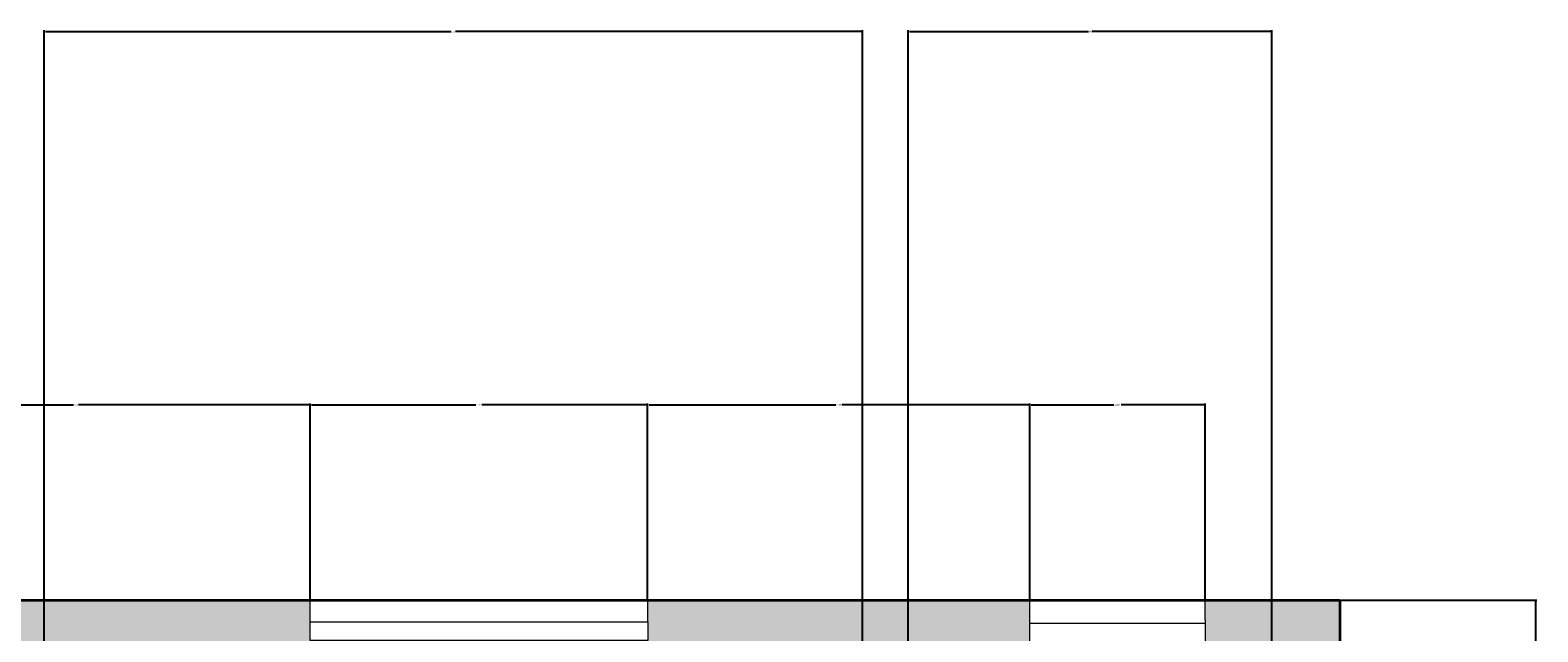
# Model space of a CAD drawing. Units: inches. Extents: x 3024 to 3952, y 1308 to 1863.
# Tile 27 of 29: x 3297 to 3496, y 1783 to 1863. Entities that reach past the tile are written whole.
import ezdxf

# ---------------------------------------------------------------- set-up
doc = ezdxf.new("R2010")
doc.units = ezdxf.units.IN
for name, color, linetype, lineweight in [('A-ANNO-DIMS', 2, 'Continuous', 18), ('A-GLAZ', 4, 'Continuous', 18), ('A-WALL', 7, 'Continuous', 35)]:
    doc.layers.add(name, color=color, linetype=linetype, lineweight=lineweight)
doc.layers.add('A-WALL-PATT', color=254, linetype='Continuous', lineweight=13, true_color=0xcecce6)
doc.styles.get("Standard").update_dxf_attribs({"font": 'arial.ttf'})
doc.dimstyles.get("Standard").update_dxf_attribs({"dimtxt": 0.18, "dimasz": 0.18, "dimexe": 0.18, "dimexo": 0.0625, "dimgap": 0.09, "dimtad": 0, "dimtih": 1, "dimtoh": 1, "dimdec": 4, "dimzin": 0, "dimdsep": 46, "dimtxsty": 'Standard', "dimcen": 0.09, "dimadec": 0, "dimazin": 0, "dimtfac": 1, "dimtdec": 4, "dimtofl": 0, "dimtmove": 0, "dimatfit": 3, "dimfxl": 1, "dimtolj": 1, "dimtzin": 0, "dimarcsym": 0})

# ---------------------------------------------------------------- blocks, each defined once
blk = doc.blocks.new('*D37')
at = {"layer": 'A-ANNO-DIMS', "color": 0, "lineweight": -2, "transparency": 16777216}
for p, q in [((3469.83, 1787.61), (3495.72, 1787.61)), ((3495.54, 1787.43), (3495.54, 1567.91)), ((3495.54, 1348.03), (3495.54, 1567.54)), ((3469.83, 1347.85), (3495.72, 1347.85))]:
    blk.add_line(p, q, dxfattribs=at)
at = {"layer": 'A-ANNO-DIMS', "color": 0, "transparency": 16777216}
for points in [[(3495.51, 1787.43), (3495.57, 1787.43), (3495.54, 1787.61)], [(3495.51, 1348.03), (3495.57, 1348.03), (3495.54, 1347.85)]]:
    blk.add_solid(points, dxfattribs=at)
at = {"layer": 'Defpoints', "color": 0, "transparency": 16777216}
for p in [(3469.76, 1787.61), (3495.54, 1787.61), (3469.76, 1347.85)]:
    blk.add_point(p, dxfattribs=at)
at = {"layer": 'A-ANNO-DIMS', "color": 0, "transparency": 16777216, "insert": (3495.54, 1567.73), "char_height": 0.18, "attachment_point": 5}
blk.add_mtext('\\A1;439.8', dxfattribs=at)
blk = doc.blocks.new('*D40')
at = {"layer": 'A-ANNO-DIMS', "color": 0, "lineweight": -2, "transparency": 16777216}
for p, q in [((3298.76, 1778.67), (3298.76, 1862.78)), ((3298.94, 1862.6), (3352.48, 1862.6)), ((3406.58, 1862.6), (3353.04, 1862.6)), ((3406.76, 1778.67), (3406.76, 1862.78))]:
    blk.add_line(p, q, dxfattribs=at)
at = {"layer": 'A-ANNO-DIMS', "color": 0, "transparency": 16777216}
for points in [[(3298.94, 1862.63), (3298.94, 1862.57), (3298.76, 1862.6)], [(3406.58, 1862.63), (3406.58, 1862.57), (3406.76, 1862.6)]]:
    blk.add_solid(points, dxfattribs=at)
at = {"layer": 'Defpoints', "color": 0, "transparency": 16777216}
for p in [(3406.76, 1862.6), (3298.76, 1778.61), (3406.76, 1778.61)]:
    blk.add_point(p, dxfattribs=at)
at = {"layer": 'A-ANNO-DIMS', "color": 0, "transparency": 16777216, "insert": (3352.76, 1862.6), "char_height": 0.18, "attachment_point": 5}
blk.add_mtext('\\A1;108', dxfattribs=at)
blk = doc.blocks.new('*D41')
at = {"layer": 'A-ANNO-DIMS', "color": 0, "lineweight": -2, "transparency": 16777216}
for p, q in [((3412.76, 1778.67), (3412.76, 1862.78)), ((3412.94, 1862.6), (3436.54, 1862.6)), ((3460.58, 1862.6), (3436.99, 1862.6)), ((3460.76, 1778.67), (3460.76, 1862.78))]:
    blk.add_line(p, q, dxfattribs=at)
at = {"layer": 'A-ANNO-DIMS', "color": 0, "transparency": 16777216}
for points in [[(3412.94, 1862.63), (3412.94, 1862.57), (3412.76, 1862.6)], [(3460.58, 1862.63), (3460.58, 1862.57), (3460.76, 1862.6)]]:
    blk.add_solid(points, dxfattribs=at)
at = {"layer": 'Defpoints', "color": 0, "transparency": 16777216}
for p in [(3460.76, 1862.6), (3412.76, 1778.61), (3460.76, 1778.61)]:
    blk.add_point(p, dxfattribs=at)
at = {"layer": 'A-ANNO-DIMS', "color": 0, "transparency": 16777216, "insert": (3436.76, 1862.6), "char_height": 0.18, "attachment_point": 5}
blk.add_mtext('\\A1;48', dxfattribs=at)
blk = doc.blocks.new('*D69')
at = {"layer": 'A-ANNO-DIMS', "color": 0, "lineweight": -2, "transparency": 16777216}
for p, q in [((3333.86, 1787.67), (3333.86, 1813.56)), ((3334.04, 1813.38), (3355.73, 1813.38)), ((3378.21, 1813.38), (3356.52, 1813.38)), ((3378.39, 1787.67), (3378.39, 1813.56))]:
    blk.add_line(p, q, dxfattribs=at)
at = {"layer": 'A-ANNO-DIMS', "color": 0, "transparency": 16777216}
for points in [[(3334.04, 1813.41), (3334.04, 1813.35), (3333.86, 1813.38)], [(3378.21, 1813.41), (3378.21, 1813.35), (3378.39, 1813.38)]]:
    blk.add_solid(points, dxfattribs=at)
at = {"layer": 'Defpoints', "color": 0, "transparency": 16777216}
for p in [(3378.39, 1813.38), (3333.86, 1787.61), (3378.39, 1787.61)]:
    blk.add_point(p, dxfattribs=at)
at = {"layer": 'A-ANNO-DIMS', "color": 0, "transparency": 16777216, "insert": (3356.13, 1813.38), "char_height": 0.18, "attachment_point": 5}
blk.add_mtext('\\A1;44.54', dxfattribs=at)
blk = doc.blocks.new('*D70')
at = {"layer": 'A-ANNO-DIMS', "color": 0, "lineweight": -2, "transparency": 16777216}
for p, q in [((3428.83, 1787.67), (3428.83, 1813.56)), ((3429.01, 1813.38), (3439.92, 1813.38)), ((3451.76, 1813.38), (3440.85, 1813.38)), ((3451.94, 1787.67), (3451.94, 1813.56))]:
    blk.add_line(p, q, dxfattribs=at)
at = {"layer": 'A-ANNO-DIMS', "color": 0, "transparency": 16777216}
for points in [[(3429.01, 1813.41), (3429.01, 1813.35), (3428.83, 1813.38)], [(3451.76, 1813.41), (3451.76, 1813.35), (3451.94, 1813.38)]]:
    blk.add_solid(points, dxfattribs=at)
at = {"layer": 'Defpoints', "color": 0, "transparency": 16777216}
for p in [(3451.94, 1813.38), (3428.83, 1787.61), (3451.94, 1787.61)]:
    blk.add_point(p, dxfattribs=at)
at = {"layer": 'A-ANNO-DIMS', "color": 0, "transparency": 16777216, "insert": (3440.39, 1813.38), "char_height": 0.18, "attachment_point": 5}
blk.add_mtext('\\A1;23.104', dxfattribs=at)
blk = doc.blocks.new('*D73')
at = {"layer": 'A-ANNO-DIMS', "color": 0, "lineweight": -2, "transparency": 16777216}
for p, q in [((3272.05, 1787.67), (3272.05, 1813.56)), ((3272.23, 1813.38), (3302.63, 1813.38)), ((3333.68, 1813.38), (3303.28, 1813.38)), ((3333.86, 1787.67), (3333.86, 1813.56))]:
    blk.add_line(p, q, dxfattribs=at)
at = {"layer": 'A-ANNO-DIMS', "color": 0, "transparency": 16777216}
for points in [[(3272.23, 1813.41), (3272.23, 1813.35), (3272.05, 1813.38)], [(3333.68, 1813.41), (3333.68, 1813.35), (3333.86, 1813.38)]]:
    blk.add_solid(points, dxfattribs=at)
at = {"layer": 'Defpoints', "color": 0, "transparency": 16777216}
for p in [(3333.86, 1813.38), (3272.05, 1787.61), (3333.86, 1787.61)]:
    blk.add_point(p, dxfattribs=at)
at = {"layer": 'A-ANNO-DIMS', "color": 0, "transparency": 16777216, "insert": (3302.95, 1813.38), "char_height": 0.18, "attachment_point": 5}
blk.add_mtext('\\A1;61.8', dxfattribs=at)
blk = doc.blocks.new('*D74')
at = {"layer": 'A-ANNO-DIMS', "color": 0, "lineweight": -2, "transparency": 16777216}
for p, q in [((3378.39, 1787.67), (3378.39, 1813.56)), ((3378.57, 1813.38), (3403.22, 1813.38)), ((3428.65, 1813.38), (3404.01, 1813.38)), ((3428.83, 1787.67), (3428.83, 1813.56))]:
    blk.add_line(p, q, dxfattribs=at)
at = {"layer": 'A-ANNO-DIMS', "color": 0, "transparency": 16777216}
for points in [[(3378.57, 1813.41), (3378.57, 1813.35), (3378.39, 1813.38)], [(3428.65, 1813.41), (3428.65, 1813.35), (3428.83, 1813.38)]]:
    blk.add_solid(points, dxfattribs=at)
at = {"layer": 'Defpoints', "color": 0, "transparency": 16777216}
for p in [(3428.83, 1813.38), (3378.39, 1787.61), (3428.83, 1787.61)]:
    blk.add_point(p, dxfattribs=at)
at = {"layer": 'A-ANNO-DIMS', "color": 0, "transparency": 16777216, "insert": (3403.61, 1813.38), "char_height": 0.18, "attachment_point": 5}
blk.add_mtext('\\A1;50.44', dxfattribs=at)

msp = doc.modelspace()

# ---------------------------------------------------------------- hatches: boundary and pattern name
at = {"layer": 'A-WALL-PATT'}
h = msp.add_hatch(color=256, dxfattribs=at)
h.dxf.hatch_style = 1
h.paths.add_polyline_path([(3106.764, 1778.6064), (3140.5977, 1778.6064), (3140.5977, 1781.8824), (3140.5977, 1784.6), (3140.5977, 1787.6064), (3097.764, 1787.6064), (3097.764, 1590.213), (3101.04, 1590.213), (3103.7576, 1590.213), (3106.764, 1590.213)])
h.paths.add_polyline_path([(3253.5314, 1781.8824), (3253.5314, 1784.6), (3253.5314, 1787.6064), (3194.6826, 1787.6064), (3194.6826, 1785.0146), (3194.6826, 1784.6), (3194.6826, 1781.8824), (3194.6826, 1778.6064), (3253.5314, 1778.6064)])
h.paths.add_polyline_path([(3333.856, 1782.2838), (3333.856, 1784.7474), (3333.856, 1787.6064), (3272.0523, 1787.6064), (3272.0523, 1785.0146), (3272.0523, 1784.6), (3272.0523, 1781.8824), (3272.0523, 1778.6064), (3333.856, 1778.6064)])
h.paths.add_polyline_path([(3428.8344, 1784.6), (3428.8344, 1787.6064), (3378.3947, 1787.6064), (3378.3947, 1784.7474), (3378.3947, 1782.2838), (3378.3947, 1778.6064), (3428.8344, 1778.6064), (3428.8344, 1781.8824)], flags=17)
h.paths.add_polyline_path([(3469.764, 1787.6064), (3451.9386, 1787.6064), (3451.9386, 1785.0146), (3451.9386, 1784.6), (3451.9386, 1781.8824), (3451.9386, 1778.6064), (3460.764, 1778.6064), (3460.764, 1353.8452), (3277.764, 1353.8452), (3277.764, 1347.8452), (3469.764, 1347.8452), (3469.764, 1353.8452)])
h.paths.add_polyline_path([(3106.764, 1571.6922), (3104.1722, 1571.6922), (3103.7576, 1571.6922), (3101.04, 1571.6922), (3097.764, 1571.6922), (3097.764, 1347.8452), (3148.7271, 1347.8452), (3148.7271, 1351.1212), (3148.7271, 1353.8388), (3148.7271, 1356.8452), (3106.764, 1356.8452)])
h.paths.add_polyline_path([(3277.764, 1532.6064), (3262.7605, 1532.6064), (3262.7605, 1582.9359), (3256.7605, 1582.9359), (3256.7605, 1532.6064), (3244.2116, 1532.6064), (3216.238, 1532.6064), (3216.238, 1527.2064), (3216.238, 1526.6064), (3271.764, 1526.6064), (3271.764, 1356.8452), (3202.812, 1356.8452), (3202.812, 1354.2534), (3202.812, 1353.8388), (3202.812, 1351.1212), (3202.812, 1347.8452), (3277.764, 1347.8452), (3277.764, 1353.8452), (3277.764, 1356.8452)])
h.paths.add_polyline_path([(3180.238, 1532.6064), (3163.0285, 1532.6064), (3163.0285, 1531.1064), (3163.0285, 1526.6064), (3180.243, 1526.6064, -0.00416688), (3180.238, 1527.2064)])
h.paths.add_polyline_path([(3133.0285, 1531.1064, -0.01250587), (3133.066, 1532.6064), (3106.764, 1532.6064), (3106.764, 1526.6064), (3133.0285, 1526.6064)], flags=17)
h.paths.add_polyline_path([(3172.764, 1628.6064), (3166.764, 1628.6064), (3166.764, 1532.6064), (3172.764, 1532.6064)])
h.paths.add_polyline_path([(3232.764, 1649.8972), (3227.364, 1649.8972), (3226.764, 1649.8972), (3226.764, 1634.6064), (3106.764, 1634.6064), (3106.764, 1628.6064), (3232.764, 1628.6064)])

# ---------------------------------------------------------------- linework, layer by layer
at = {"layer": 'A-GLAZ'}
for p, q in [((3333.856, 1784.7474), (3333.856, 1787.6064)), ((3378.3947, 1784.7474), (3378.3947, 1787.6064)), ((3428.8344, 1784.6), (3428.8344, 1787.6064)), ((3451.9386, 1785.0146), (3451.9386, 1787.6064)), ((3451.9386, 1785.0146), (3451.9386, 1784.6))]:
    msp.add_line(p, q, dxfattribs=at)
for points in [[(3333.856, 1784.7474), (3378.3947, 1784.7474), (3378.3947, 1782.2838), (3333.856, 1782.2838)], [(3428.8344, 1784.6), (3451.9386, 1784.6), (3451.9386, 1781.8824), (3428.8344, 1781.8824)]]:
    msp.add_lwpolyline(points, close=True, dxfattribs=at)
at = {"layer": 'A-WALL'}
for p in [(3097.764, 1787.6064), (3469.764, 1347.8452)]:
    msp.add_line(p, (3469.764, 1787.6064), dxfattribs=at)

# ---------------------------------------------------------------- dimensions: what is measured, and where the dimension line sits
at = {"layer": 'A-ANNO-DIMS'}
for base, p1, p2, override, picture, middle in [((3406.764, 1862.6031), (3298.764, 1778.6064), (3406.764, 1778.6064), {"dimdec": 0, "dimlfac": 1, "dimrnd": 0, "dimzin": 0, "dimdsep": 46, "dimlunit": 2}, '*D40', (3352.764, 1862.6031)), ((3460.764, 1862.6031), (3412.764, 1778.6064), (3460.764, 1778.6064), {"dimdec": 0, "dimlfac": 1, "dimrnd": 0, "dimzin": 0, "dimdsep": 46, "dimlunit": 2}, '*D41', (3436.764, 1862.6031)), ((3333.856, 1813.3814), (3272.0523, 1787.6064), (3333.856, 1787.6064), {"dimdec": 1, "dimlfac": 1, "dimrnd": 0, "dimzin": 0, "dimdsep": 46, "dimlunit": 2}, '*D73', (3302.9541, 1813.3814)), ((3378.3947, 1813.3814), (3333.856, 1787.6064), (3378.3947, 1787.6064), {"dimdec": 2, "dimlfac": 1, "dimrnd": 0, "dimzin": 0, "dimdsep": 46, "dimlunit": 2}, '*D69', (3356.1254, 1813.3814)), ((3428.8344, 1813.3814), (3378.3947, 1787.6064), (3428.8344, 1787.6064), {"dimdec": 2, "dimlfac": 1, "dimrnd": 0, "dimzin": 0, "dimdsep": 46, "dimlunit": 2}, '*D74', (3403.6146, 1813.3814)), ((3451.9386, 1813.3814), (3428.8344, 1787.6064), (3451.9386, 1787.6064), {"dimdec": 3, "dimlfac": 1, "dimrnd": 0, "dimzin": 0, "dimdsep": 46, "dimlunit": 2}, '*D70', (3440.3865, 1813.3814))]:
    dim = msp.add_linear_dim(base=base, p1=p1, p2=p2, dimstyle='Standard', override=override, dxfattribs=at)
    dim.commit()
    dim.dimension.update_dxf_attribs({"geometry": picture, "text_midpoint": middle})
dim = msp.add_linear_dim(base=(3495.539, 1787.6064), p1=(3469.764, 1347.8452), p2=(3469.764, 1787.6064), angle=90, dimstyle='Standard', override={"dimdec": 1, "dimlfac": 1, "dimrnd": 0, "dimzin": 0, "dimdsep": 46, "dimlunit": 2}, dxfattribs=at)
dim.commit()
dim.dimension.update_dxf_attribs({"geometry": '*D37', "text_midpoint": (3495.539, 1567.7258)})

doc.saveas('drawing.dxf')
